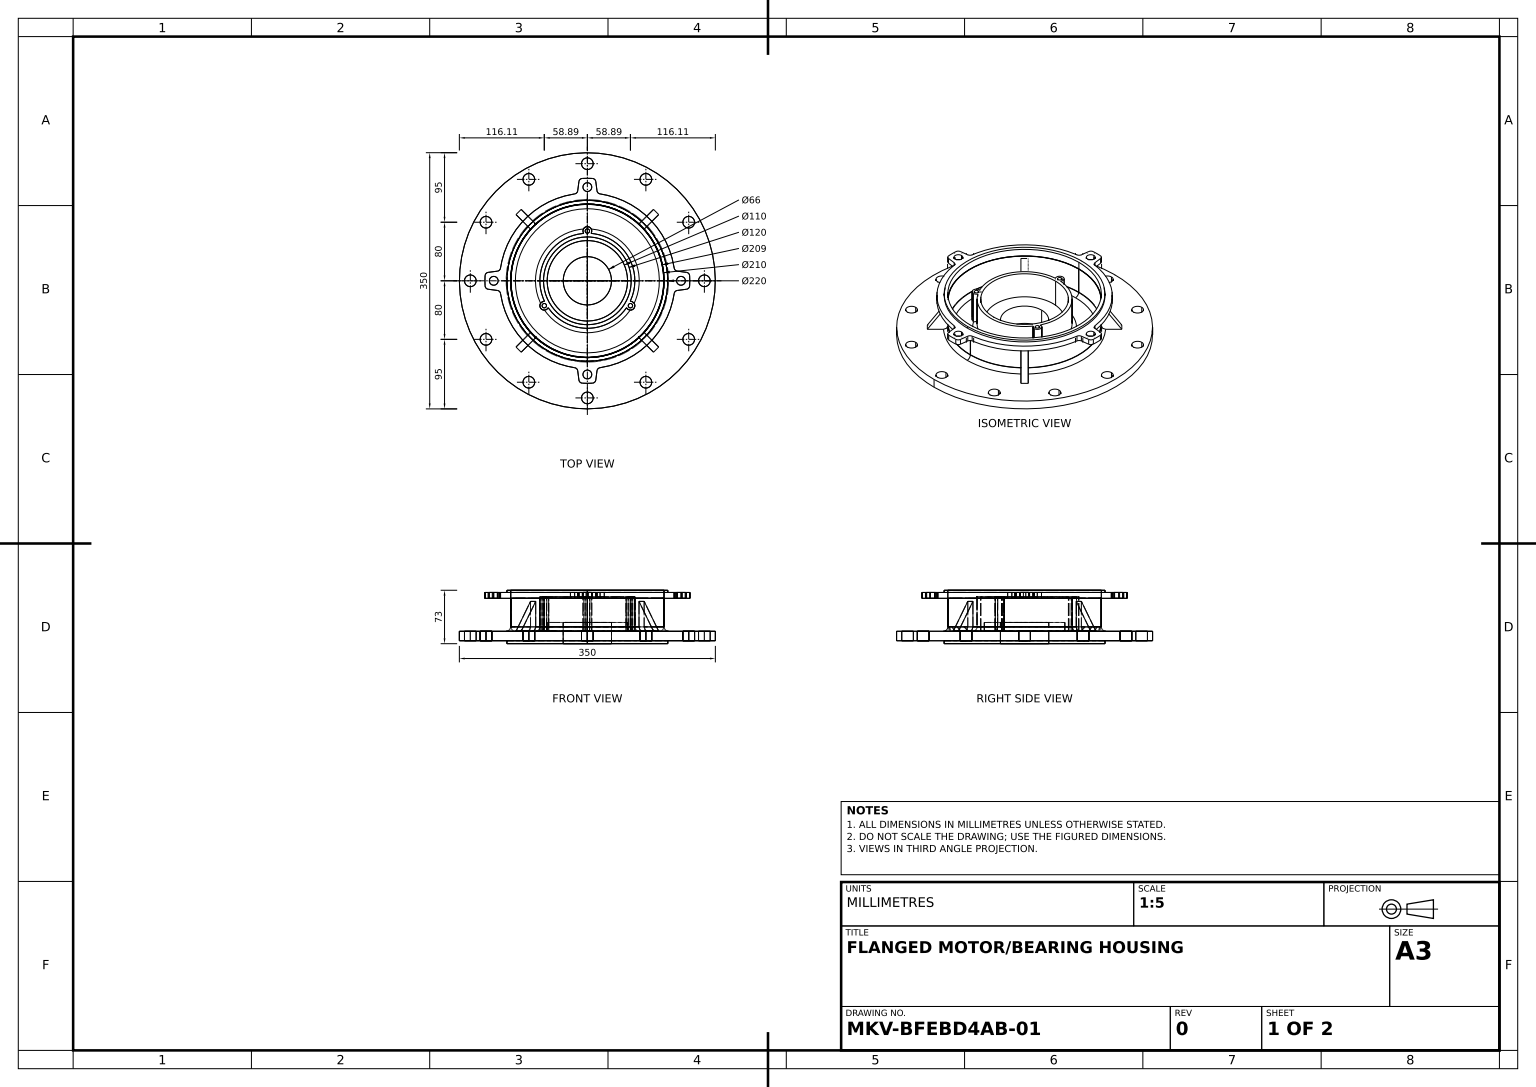
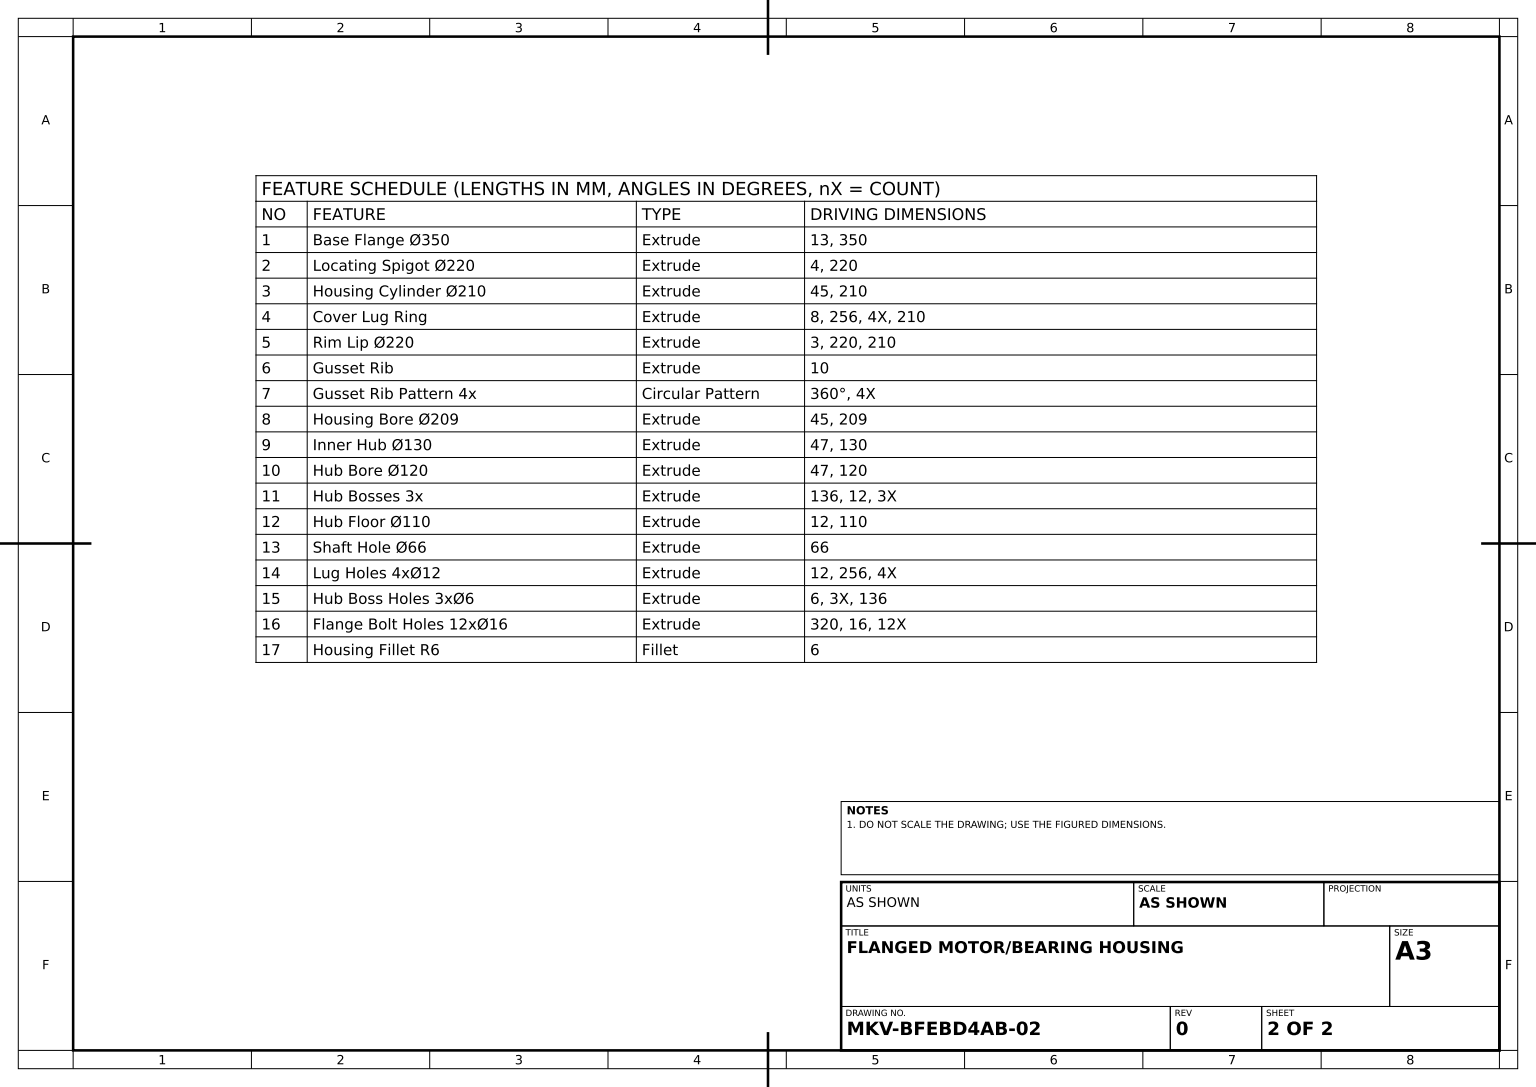
SolidWorks part; units mm, degrees
material "Plain Carbon Steel"
ref_plane "Front Plane" through (0, 0, 0) normal (0, 0, 1) x (1, 0, 0)
ref_plane "Top Plane" through (0, 0, 0) normal (0, 1, 0) x (1, 0, 0)
ref_plane "Right Plane" through (0, 0, 0) normal (1, 0, 0) x (0, 0, -1)
sketch "Flange Sketch Ø350" plane through (0, 0, 0) normal (0, 1, 0) x (1, 0, 0)
  circle A0 centre (0, 0) radius 175
  dimension "D1" = 350
extrude "Base Flange Ø350" add sketch "Flange Sketch Ø350" along normal blind 13
sketch "Spigot Sketch Ø220" plane through (0, 0, 0) normal (0, -1, 0) x (1, 0, 0)
  circle A0 centre (0, 0) radius 110
  dimension "D1" = 220
extrude "Locating Spigot Ø220" add sketch "Spigot Sketch Ø220" along normal blind 4
sketch "Housing Sketch Ø210" plane through (0, 13, 0) normal (0, 1, 0) x (1, 0, 0)
  circle A0 centre (0, 0) radius 105
  dimension "D1" = 210
extrude "Housing Cylinder Ø210" add sketch "Housing Sketch Ø210" along normal blind 45
sketch "Lug Ring Sketch" plane through (0, 58, 0) normal (0, 1, 0) x (1, 0, 0)
  line L0 (135.4922, 11.5365) -> (123.0249, 13.1778)
  line L1 (135.4922, -11.5365) -> (123.0249, -13.1778)
  line L2 (11.5365, -135.4922) -> (13.1778, -123.0249)
  line L3 (-11.5365, 135.4922) -> (-13.1778, 123.0249)
  line L4 (11.5365, 135.4922) -> (13.1778, 123.0249)
  line L5 (-11.5365, -135.4922) -> (-13.1778, -123.0249)
  line L6 (-135.4922, -11.5365) -> (-123.0249, -13.1778)
  line L7 (-135.4922, 11.5365) -> (-123.0249, 13.1778)
  arc A0 (-17.4097, 118.7304) -> (-118.7304, 17.4097) centre (0, 0) ccw
  arc A2 (6.8229, 139.8336) -> (-6.8229, 139.8336) centre (0, 0) ccw
  circle A3 centre (0, 0) radius 128 construction
  arc A4 (-11.5365, 135.4922) -> (-6.8229, 139.8336) centre (-6.5793, 134.8396) cw
  arc A5 (6.8229, 139.8336) -> (11.5365, 135.4922) centre (6.5793, 134.8396) cw
  arc A6 (-13.1778, 123.0249) -> (-17.4097, 118.7304) centre (-18.1351, 123.6775) cw
  arc A7 (13.1778, 123.0249) -> (17.4097, 118.7304) centre (18.1351, 123.6775) ccw
  arc A8 (135.4922, 11.5365) -> (139.8336, 6.8229) centre (134.8396, 6.5793) cw
  arc A9 (123.0249, 13.1778) -> (118.7304, 17.4097) centre (123.6775, 18.1351) cw
  arc A10 (139.8336, -6.8229) -> (139.8336, 6.8229) centre (0, 0) ccw
  arc A11 (139.8336, -6.8229) -> (135.4922, -11.5365) centre (134.8396, -6.5793) cw
  arc A12 (123.0249, -13.1778) -> (118.7304, -17.4097) centre (123.6775, -18.1351) ccw
  arc A13 (11.5365, -135.4922) -> (6.8229, -139.8336) centre (6.5793, -134.8396) cw
  arc A14 (13.1778, -123.0249) -> (17.4097, -118.7304) centre (18.1351, -123.6775) cw
  arc A15 (-6.8229, -139.8336) -> (6.8229, -139.8336) centre (0, 0) ccw
  arc A16 (-6.8229, -139.8336) -> (-11.5365, -135.4922) centre (-6.5793, -134.8396) cw
  arc A17 (-13.1778, -123.0249) -> (-17.4097, -118.7304) centre (-18.1351, -123.6775) ccw
  arc A18 (-135.4922, -11.5365) -> (-139.8336, -6.8229) centre (-134.8396, -6.5793) cw
  arc A19 (-123.0249, -13.1778) -> (-118.7304, -17.4097) centre (-123.6775, -18.1351) cw
  arc A20 (-139.8336, 6.8229) -> (-139.8336, -6.8229) centre (0, 0) ccw
  arc A21 (-139.8336, 6.8229) -> (-135.4922, 11.5365) centre (-134.8396, 6.5793) cw
  arc A22 (-123.0249, 13.1778) -> (-118.7304, 17.4097) centre (-123.6775, 18.1351) ccw
  arc A23 (-118.7304, -17.4097) -> (-17.4097, -118.7304) centre (0, 0) ccw
  arc A24 (17.4097, -118.7304) -> (118.7304, -17.4097) centre (0, 0) ccw
  arc A25 (118.7304, 17.4097) -> (17.4097, 118.7304) centre (0, 0) ccw
  circle A26 centre (0, 0) radius 105
  dimension "D1" = 210
  dimension "D2" = 120
  dimension "D3" = 4
  dimension "D4" = 256
  dimension "D5" = 140
  dimension "D6" = 5
  dimension "D7" = 13.6459
  dimension "D8" = 15
extrude "Cover Lug Ring" add sketch "Lug Ring Sketch" along normal blind 8 separate body
sketch "Rim Lip Sketch" plane through (0, 66, 0) normal (0, 1, 0) x (1, 0, 0)
  circle A0 centre (0, 0) radius 110
  circle A1 centre (0, 0) radius 105
  dimension "D1" = 220
  dimension "D2" = 210
extrude "Rim Lip Ø220" add sketch "Rim Lip Sketch" along normal blind 3
sketch "Rib Plane Line 45deg" plane through (0, 13, 0) normal (0, 1, 0) x (1, 0, 0)
  line L0 (0, 0) -> (-107.0345, 107.0345) construction
  dimension "D1" = 45
ref_plane "Rib Plane" through (0, 0, 0) normal (0.7071, 0, -0.7071) x (-0.7071, 0, -0.7071)
sketch "Gusset Rib Profile" plane through (0, 0, 0) normal (0.7071, 0, -0.7071) x (-0.7071, 0, -0.7071)
  line L0 (102.9385, 56.6059) -> (102.9385, 13)
  line L1 (0, 13) -> (151.3696, 13) construction
  line L2 (102.9385, 13) -> (132.9385, 13)
  line L3 (132.9385, 13) -> (102.9385, 56.6059)
  dimension "D1" = 43.6059
  dimension "D2" = 30
  dimension "D3" = 102.9385
extrude "Gusset Rib" add sketch "Gusset Rib Profile" along normal mid plane 10
pattern_circular "Gusset Rib Pattern 4x" count 4 over 360 about axis through (0, 0, 0) along (0, 1, 0) of "Gusset Rib"
sketch "Housing Bore Sketch Ø209" plane through (0, 58, 0) normal (0, 1, 0) x (1, 0, 0)
  circle A0 centre (0, 0) radius 104.5
  dimension "D1" = 209
extrude "Housing Bore Ø209" cut sketch "Housing Bore Sketch Ø209" against normal blind 45
sketch "Hub Sketch Ø130" plane through (0, 13, 0) normal (0, 1, 0) x (1, 0, 0)
  circle A0 centre (0, 0) radius 65
  dimension "D1" = 130
extrude "Inner Hub Ø130" add sketch "Hub Sketch Ø130" along normal blind 47
sketch "Hub Bore Sketch Ø120" plane through (0, 60, 0) normal (0, 1, 0) x (1, 0, 0)
  circle A0 centre (0, 0) radius 60
  dimension "D1" = 120
extrude "Hub Bore Ø120" cut sketch "Hub Bore Sketch Ø120" against normal blind 47
sketch "Hub Bosses Sketch 3x" plane through (0, 60, 0) normal (0, 1, 0) x (1, 0, 0)
  circle A0 centre (0, 0) radius 68 construction
  circle A1 centre (0, 68) radius 6
  circle A2 centre (58.8897, -34) radius 6
  circle A3 centre (-58.8897, -34) radius 6
  dimension "D1" = 136
  dimension "D2" = 12
  dimension "D3" = 3
extrude "Hub Bosses 3x" add sketch "Hub Bosses Sketch 3x" against normal up to next
sketch "Hub Floor Sketch Ø110" plane through (0, 13, 0) normal (0, 1, 0) x (1, 0, 0)
  circle A0 centre (0, 0) radius 55
  dimension "D1" = 110
extrude "Hub Floor Ø110" add sketch "Hub Floor Sketch Ø110" along normal blind 12
sketch "Shaft Hole Sketch Ø66" plane through (0, 25, 0) normal (0, 1, 0) x (1, 0, 0)
  circle A0 centre (0, 0) radius 33
  dimension "D1" = 66
extrude "Shaft Hole Ø66" cut sketch "Shaft Hole Sketch Ø66" against normal up to next (29 mm away)
sketch "Lug Holes Sketch 4xØ12" plane through (0, 66, 0) normal (0, 1, 0) x (1, 0, 0)
  circle A0 centre (0, 0) radius 128 construction
  circle A1 centre (0, 128) radius 6
  circle A2 centre (128, 0) radius 6
  circle A3 centre (0, -128) radius 6
  circle A4 centre (-128, 0) radius 6
  dimension "D1" = 256
  dimension "D2" = 12
  dimension "D3" = 4
extrude "Lug Holes 4xØ12" cut sketch "Lug Holes Sketch 4xØ12" against normal blind 12
sketch "Boss Holes Sketch 3xØ6" plane through (0, 60, 0) normal (0, 1, 0) x (1, 0, 0)
  circle A0 centre (0, 68) radius 3
  circle A1 centre (58.8897, -34) radius 3
  circle A2 centre (-58.8897, -34) radius 3
  circle A3 centre (0, 0) radius 68 construction
  dimension "D1" = 6
  dimension "D3" = 136
  dimension "D2" = 3
extrude "Hub Boss Holes 3xØ6" cut sketch "Boss Holes Sketch 3xØ6" against normal up to surface (47 mm away) up to face at (0, 13, 0)
sketch "Bolt Holes Sketch 12xØ16" plane through (0, 13, 0) normal (0, 1, 0) x (1, 0, 0)
  circle A0 centre (0, 0) radius 160 construction
  circle A1 centre (0, 160) radius 8
  circle A2 centre (80, 138.5641) radius 8
  circle A3 centre (138.5641, 80) radius 8
  circle A4 centre (160, 0) radius 8
  circle A5 centre (138.5641, -80) radius 8
  circle A6 centre (80, -138.5641) radius 8
  circle A7 centre (0, -160) radius 8
  circle A8 centre (-80, -138.5641) radius 8
  circle A9 centre (-138.5641, -80) radius 8
  circle A10 centre (-160, 0) radius 8
  circle A11 centre (-138.5641, 80) radius 8
  circle A12 centre (-80, 138.5641) radius 8
  dimension "D1" = 320
  dimension "D2" = 16
  dimension "D3" = 12
extrude "Flange Bolt Holes 12xØ16" cut sketch "Bolt Holes Sketch 12xØ16" against normal up to next (13 mm away)
fillet "Housing Fillet R6" radius 6 8 edges at (56.2917, 13, -32.5) (0, 13, 65) (-56.2917, 13, -32.5) (0, 13, 104.5) (0, 13, -105) (105, 13, 0) (-105, 13, 0) (0, 13, 105)
